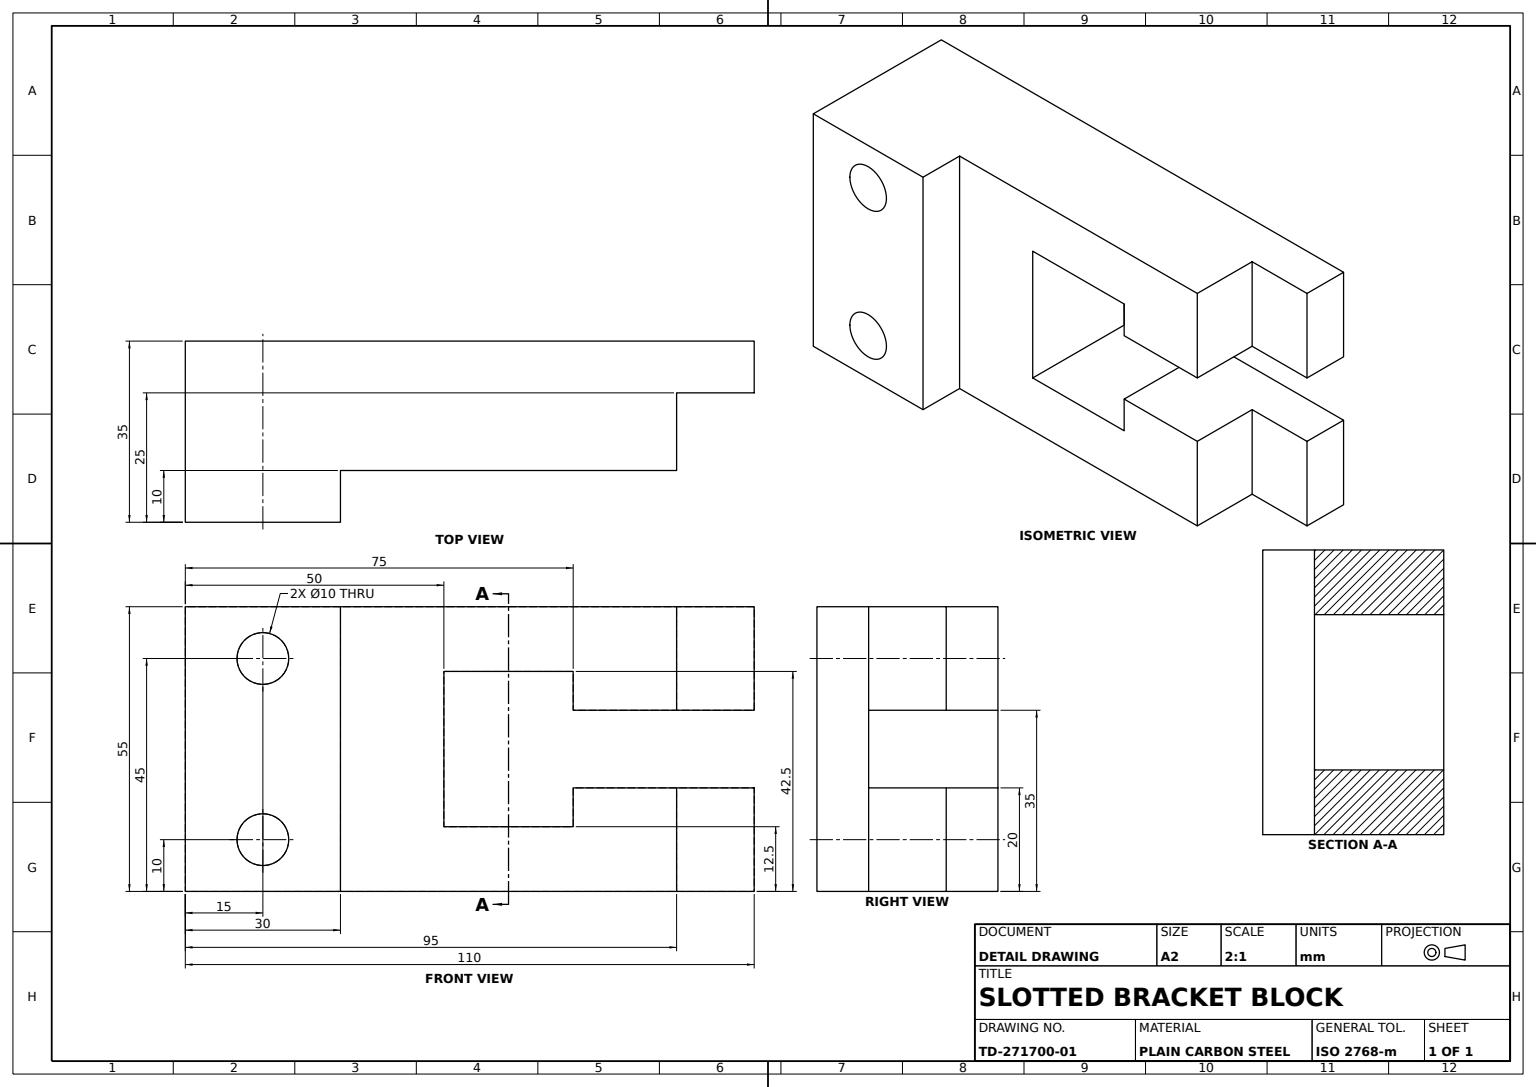
from build123d import *

# Parameters (mm, degrees)
BASE_PROFILE_DEPTH     = 10
UPRIGHT_BLOCK_SKETCH_W = 30
UPRIGHT_BLOCK_SKETCH_H = 55
UPRIGHT_BLOCK_DEPTH    = 25
SLOTTED_ARM_DEPTH      = 15
THROUGH_HOLES_SKETCH_R = 5
THROUGH_HOLES_2X_DEPTH = 55


with BuildPart() as part:
    # Base Profile Sketch → Base Profile (new body)
    with BuildSketch(Plane.XY):
        Polygon((0, 0), (0, -55), (110, -55), (110, -35), (75, -35), (75, -42.5), (50, -42.5), (50, -12.5), (75, -12.5), (75, -20), (110, -20), (110, 0), align=None)
    extrude(amount=BASE_PROFILE_DEPTH)

    # Upright Block Sketch → Upright Block (add)
    with BuildSketch(Plane.XY.offset(10)):
        with Locations((15, -27.5)):
            Rectangle(UPRIGHT_BLOCK_SKETCH_W, UPRIGHT_BLOCK_SKETCH_H)
    extrude(amount=UPRIGHT_BLOCK_DEPTH)

    # Slotted Arm Sketch → Slotted Arm (add)
    with BuildSketch(Plane.XY.offset(10)):
        Polygon((30, 0), (30, -55), (95, -55), (95, -35), (75, -35), (75, -42.5), (50, -42.5), (50, -12.5), (75, -12.5), (75, -20), (95, -20), (95, 0), align=None)
    extrude(amount=SLOTTED_ARM_DEPTH)

    # Through Holes Sketch → Through Holes 2x (cut)
    with BuildSketch(Plane.XY.offset(35)):
        with Locations((15, -10)):
            Circle(THROUGH_HOLES_SKETCH_R)
        with Locations((15, -45)):
            Circle(THROUGH_HOLES_SKETCH_R)
    extrude(amount=-THROUGH_HOLES_2X_DEPTH, mode=Mode.SUBTRACT)


solid = part.part
